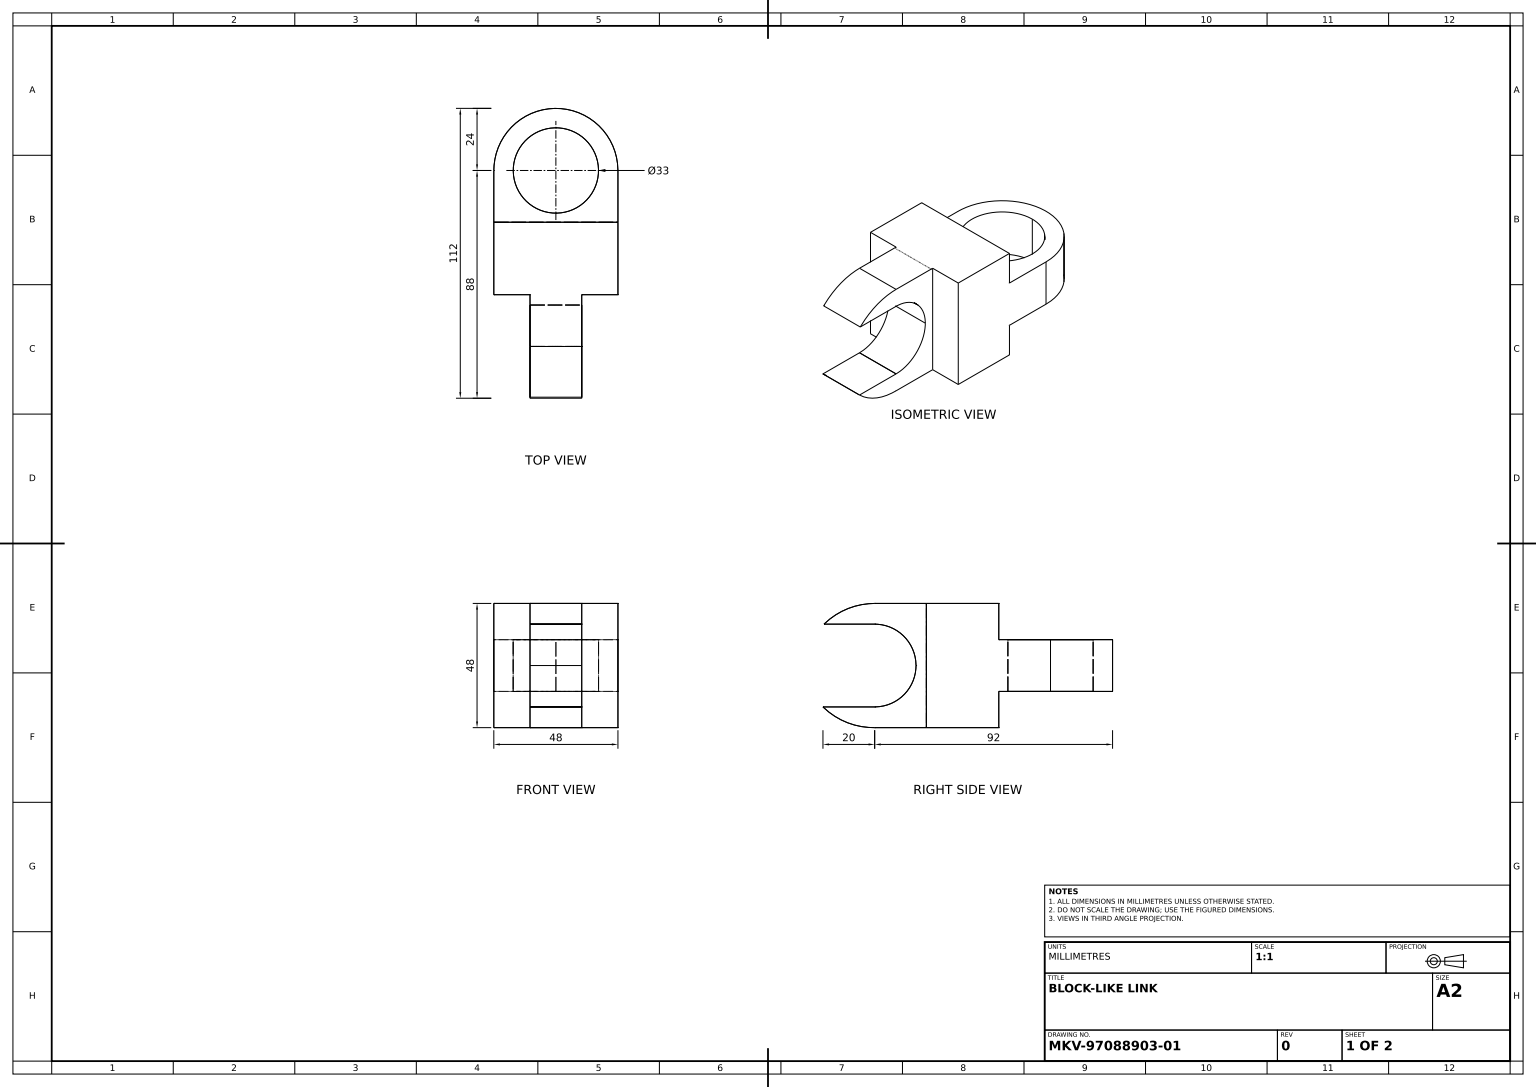
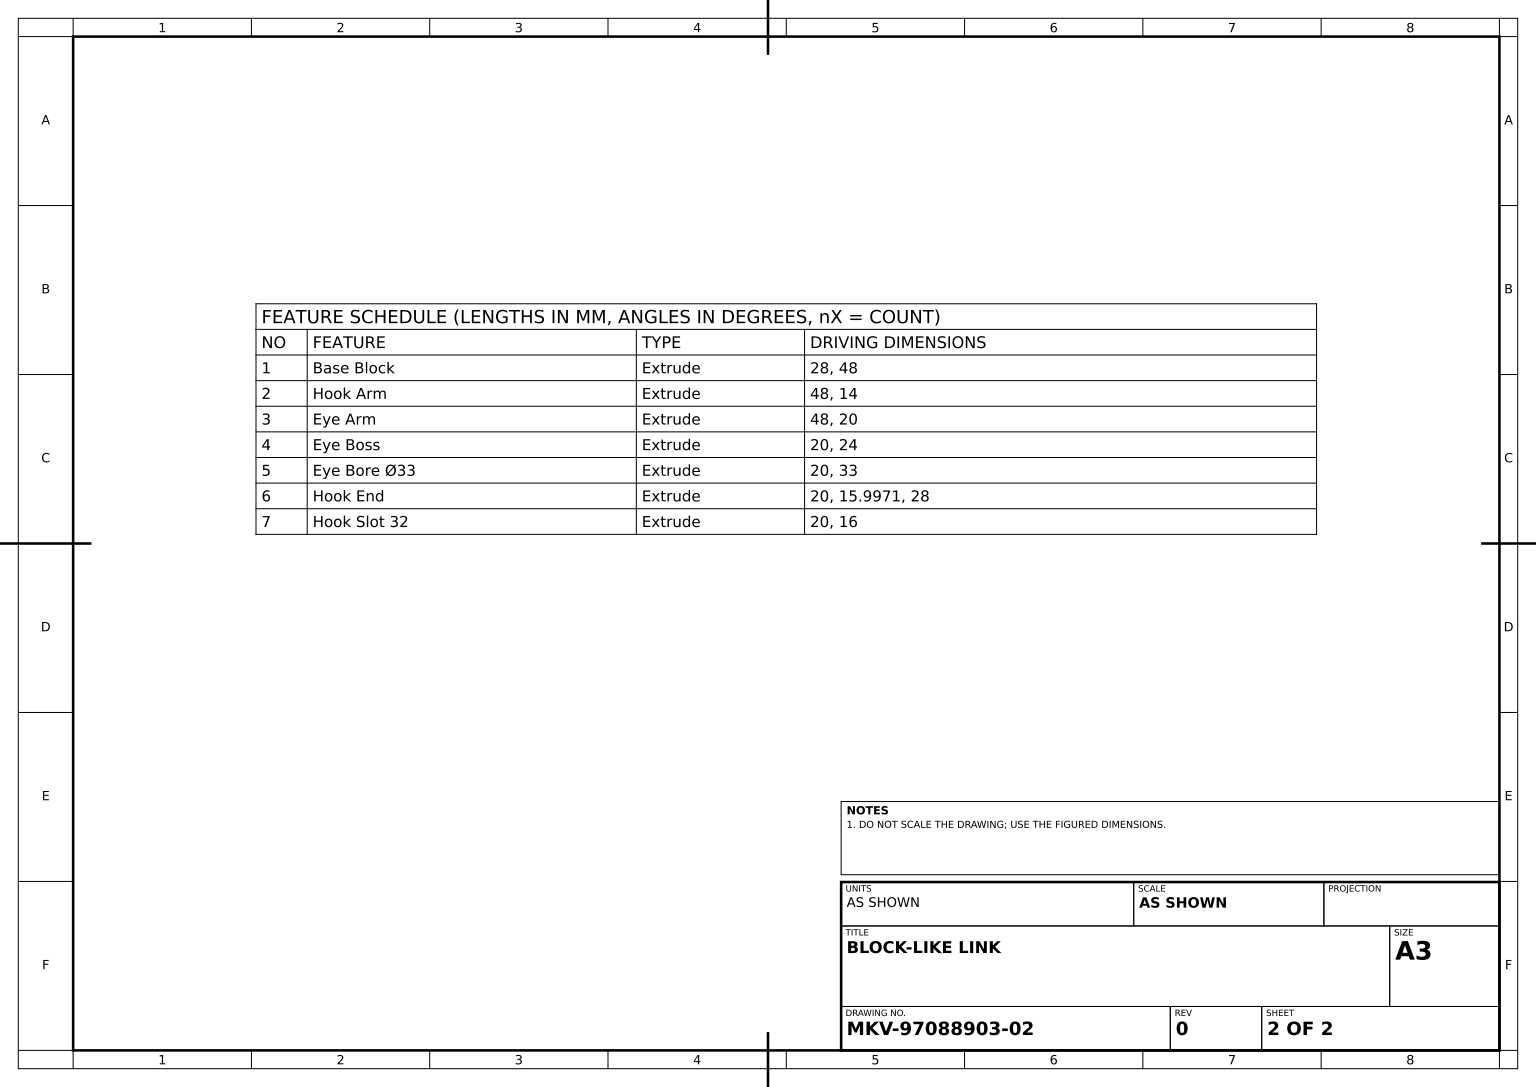
SolidWorks part; units mm, degrees
material "Plain Carbon Steel"
ref_plane "Front Plane" through (0, 0, 0) normal (0, 0, 1) x (1, 0, 0)
ref_plane "Top Plane" through (0, 0, 0) normal (0, 1, 0) x (1, 0, 0)
ref_plane "Right Plane" through (0, 0, 0) normal (1, 0, 0) x (0, 0, -1)
sketch "Base Block Sketch" plane through (0, 0, 0) normal (0, 0, 1) x (1, 0, 0)
  line L0 (0, 0) -> (48, 0)
  line L1 (48, 0) -> (48, -48)
  line L2 (48, -48) -> (0, -48)
  line L3 (0, -48) -> (0, 0)
  dimension "D1" = 48
extrude "Base Block" add sketch "Base Block Sketch" along normal blind 28
sketch "Hook Arm Sketch" plane through (0, 0, 0) normal (0, 1, 0) x (1, 0, 0)
  line L0 (24, -28) -> (14, -28)
  line L1 (48, -28) -> (0, -28) construction
  line L2 (14, -28) -> (34, -28)
  line L3 (34, -28) -> (34, -48)
  line L4 (34, -48) -> (14, -48)
  line L5 (14, -48) -> (14, -28)
  line L6 (0, -28) -> (0, 0) construction
  line M3 (0, -28) -> (48, -28)
  dimension "D1" = 14
extrude "Hook Arm" add sketch "Hook Arm Sketch" against normal blind 48 contours L5 L4 L3 M3
sketch "Eye Arm Sketch" plane through (48, 0, 0) normal (1, 0, 0) x (0, 0, -1)
  line L0 (0, -24) -> (0, -14)
  line L1 (0, -48) -> (0, 0) construction
  line L2 (0, -24) -> (0, -34)
  line L3 (0, -34) -> (20, -34)
  line L4 (20, -34) -> (20, -14)
  line L5 (20, -14) -> (0, -14)
  dimension "D1" = 20
extrude "Eye Arm" add sketch "Eye Arm Sketch" against normal blind 48
sketch "Eye Boss Sketch" plane through (0, -14, 0) normal (0, 1, 0) x (1, 0, 0)
  line L0 (0, 20) -> (48, 20) construction
  line L1 (0, 20) -> (48, 20)
  arc A0 (48, 20) -> (0, 20) centre (24, 20) ccw
  dimension "D1" = 48
  dimension "D2" = 24
extrude "Eye Boss" add sketch "Eye Boss Sketch" against normal blind 20
sketch "Eye Bore Sketch" plane through (0, -14, 0) normal (0, 1, 0) x (1, 0, 0)
  circle A0 centre (24, 20) radius 16.5
  dimension "D1" = 33
  dimension "D2" = 33
extrude "Eye Bore Ø33" cut sketch "Eye Bore Sketch" against normal blind 20
sketch "Hook End Sketch" plane through (34, 0, 0) normal (1, 0, 0) x (0, 0, -1)
  line L0 (-48, -48) -> (-48, 0) construction
  line L1 (-48, -8.0029) -> (-67.5989, -8.0029)
  line L2 (-48, -39.9971) -> (-68, -39.9971)
  line L3 (-48, -48) -> (-28, -48)
  line L4 (-48, 0) -> (-48, -48)
  arc A0 (-48, -39.9971) -> (-48, -8.0029) centre (-48, -24) ccw
  arc A1 (-67.5989, -8.0029) -> (-48, 0) centre (-48, -28) cw
  arc A2 (-68, -39.9971) -> (-48, -48) centre (-48.3983, -20.0028) ccw
  line M3 (-48, 0) -> (-48, -48)
  dimension "D1" = 31.9943
  dimension "D2" = 28
  dimension "D3" = 28
  dimension "D4" = 15.9971
  dimension "D5" = 28
extrude "Hook End" add sketch "Hook End Sketch" against normal blind 20 contours A1 L1 M3 | L2 A2 M3
sketch "Hook Slot Sketch" plane through (34, 0, 0) normal (1, 0, 0) x (0, 0, -1)
  line L0 (-48, -39.9971) -> (-48, -8.0029) construction
  line L1 (-48, -8.0029) -> (-48, -8)
  line L2 (-48, -8) -> (-48, -8.0029)
  line L3 (-48, -8.0029) -> (-48, -40)
  arc A0 (-48, -40) -> (-48, -8) centre (-48, -24) ccw
  line M4 (-48, -8.0029) -> (-48, -39.9971)
  dimension "D1" = 32
  dimension "D2" = 16
extrude "Hook Slot 32" cut sketch "Hook Slot Sketch" against normal blind 20 contours L3 A0 L1 M4
